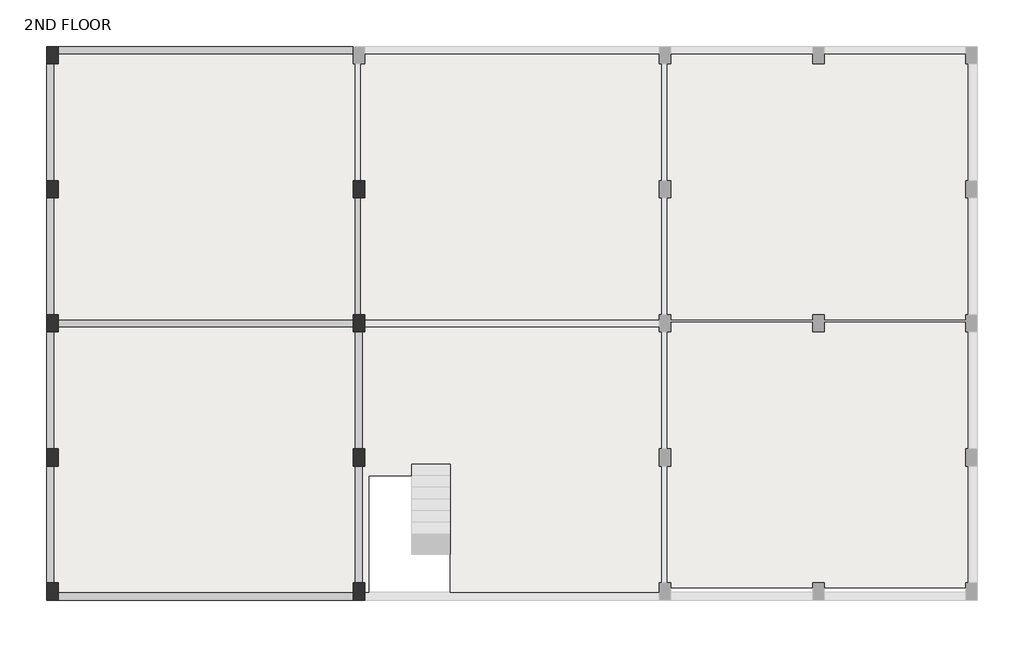
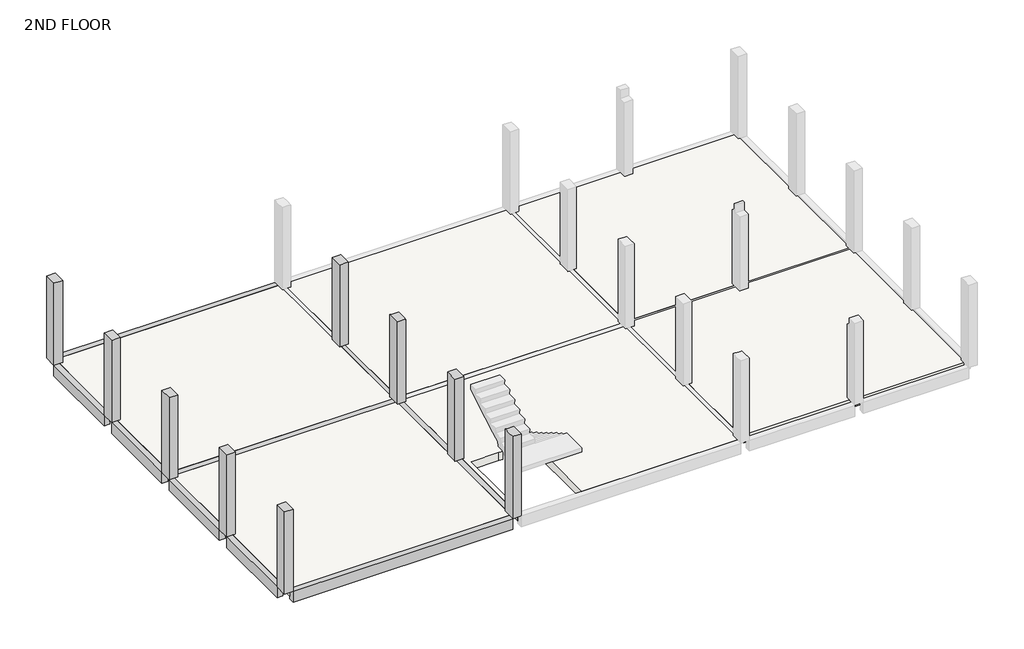
# One storey, part 1 of 2: 10 beams, 9 columns, 1 slab.
"""IFC4 building model written with IfcOpenShell, lengths in millimetres."""

from ifc_helpers import new_model, si_unit, origin, place, context, project, spatial, faceted_brep, element, save

model = new_model("IFC4")

# Units and contexts
model_context = context("Model", 3, world=origin())
ifc_project = project(units=[si_unit("LENGTHUNIT", "METRE", prefix="MILLI")], contexts=[model_context])

# Site, building, storey
site = spatial("IfcSite", under=ifc_project)
building = spatial("IfcBuilding", under=site)
storey = spatial("IfcBuildingStorey", under=building, Name="2ND FLOOR", Elevation=6096.0)

# Beams
placement = place(None, origin())
element("IfcBeam", 1, ObjectType="M_Concrete-Rectangular Beam : 200MMX400MM", at=placement, inside=storey, context=model_context, shape_type="Brep", body=[
    faceted_brep([(-3980.6874017, 15797.7008557, 6096.0), (-3980.6874017, 15997.7008557, 6096.0), (-11680.6874017, 15997.7008557, 6096.0), (-11680.6874017, 15797.7008557, 6096.0), (-3980.6874017, 15797.7008557, 5696.0), (-3980.6874017, 15797.7008557, 5796.0), (-11680.6874017, 15797.7008557, 5796.0), (-11680.6874017, 15797.7008557, 5696.0), (-3980.6874017, 15997.7008557, 5696.0), (-11680.6874017, 15997.7008557, 5696.0)], [[[0, 1, 2, 3]], [[4, 5, 0, 3, 6, 7]], [[8, 4, 7, 9]], [[1, 8, 9, 2]], [[2, 9, 7, 6, 3]], [[1, 0, 5, 4, 8]]]),
])
element("IfcBeam", 2, ObjectType="M_Concrete-Rectangular Beam : 200MMX400MM", at=placement, inside=storey, context=model_context, shape_type="Brep", body=[
    faceted_brep([(-11680.6874017, 1747.7008557, 6096.0), (-11680.6874017, 1547.7008557, 6096.0), (-3980.6874017, 1547.7008557, 6096.0), (-3980.6874017, 1747.7008557, 6096.0), (-11680.6874017, 1747.7008557, 5696.0), (-11680.6874017, 1747.7008557, 5796.0), (-3980.6874017, 1747.7008557, 5796.0), (-3980.6874017, 1747.7008557, 5696.0), (-11680.6874017, 1547.7008557, 5696.0), (-3980.6874017, 1547.7008557, 5696.0)], [[[0, 1, 2, 3]], [[4, 5, 0, 3, 6, 7]], [[8, 4, 7, 9]], [[1, 8, 9, 2]], [[1, 0, 5, 4, 8]], [[2, 9, 7, 6, 3]]]),
])
element("IfcBeam", 3, ObjectType="M_Concrete-Rectangular Beam : 200MMX400MM", at=placement, inside=storey, context=model_context, shape_type="Brep", body=[
    faceted_brep([(-3980.6874017, 8872.7008557, 6096.0), (-11680.6874017, 8872.7008557, 6096.0), (-11680.6874017, 8672.7008557, 6096.0), (-3980.6874017, 8672.7008557, 6096.0), (-11680.6874017, 8672.7008557, 5796.0), (-11680.6874017, 8672.7008557, 5696.0), (-3980.6874017, 8672.7008557, 5696.0), (-3980.6874017, 8672.7008557, 5796.0), (-11680.6874017, 8872.7008557, 5696.0), (-3980.6874017, 8872.7008557, 5696.0), (-3980.6874017, 8872.7008557, 5796.0), (-11680.6874017, 8872.7008557, 5796.0)], [[[0, 1, 2, 3]], [[3, 2, 4, 5, 6, 7]], [[6, 5, 8, 9]], [[1, 0, 10, 9, 8, 11]], [[8, 5, 4, 2, 1, 11]], [[0, 3, 7, 6, 9, 10]]]),
])
element("IfcBeam", 4, ObjectType="M_Concrete-Rectangular Beam : 200MMX400MM", at=placement, inside=storey, context=model_context, shape_type="Brep", body=[
    faceted_brep([(-11980.6874017, 12497.7008557, 6096.0), (-11780.6874017, 12497.7008557, 6096.0), (-11780.6874017, 15547.7008557, 6096.0), (-11980.6874017, 15547.7008557, 6096.0), (-11980.6874017, 12497.7008557, 5696.0), (-11980.6874017, 15547.7008557, 5696.0), (-11780.6874017, 12497.7008557, 5696.0), (-11780.6874017, 15547.7008557, 5696.0), (-11780.6874017, 12497.7008557, 5796.0), (-11780.6874017, 15547.7008557, 5796.0)], [[[0, 1, 2, 3]], [[4, 0, 3, 5]], [[6, 4, 5, 7]], [[1, 8, 6, 7, 9, 2]], [[2, 9, 7, 5, 3]], [[1, 0, 4, 6, 8]]]),
])
element("IfcBeam", 5, ObjectType="M_Concrete-Rectangular Beam : 200MMX400MM", at=placement, inside=storey, context=model_context, shape_type="Brep", body=[
    faceted_brep([(-11980.6874017, 8997.7008557, 6096.0), (-11780.6874017, 8997.7008557, 6096.0), (-11780.6874017, 12047.7008557, 6096.0), (-11980.6874017, 12047.7008557, 6096.0), (-11980.6874017, 8997.7008557, 5696.0), (-11980.6874017, 12047.7008557, 5696.0), (-11780.6874017, 8997.7008557, 5696.0), (-11780.6874017, 12047.7008557, 5696.0), (-11780.6874017, 8997.7008557, 5796.0), (-11780.6874017, 12047.7008557, 5796.0)], [[[0, 1, 2, 3]], [[4, 0, 3, 5]], [[6, 4, 5, 7]], [[1, 8, 6, 7, 9, 2]], [[1, 0, 4, 6, 8]], [[2, 9, 7, 5, 3]]]),
])
element("IfcBeam", 6, ObjectType="M_Concrete-Rectangular Beam : 200MMX400MM", at=placement, inside=storey, context=model_context, shape_type="Brep", body=[
    faceted_brep([(-11980.6874017, 5497.7008557, 6096.0), (-11780.6874017, 5497.7008557, 6096.0), (-11780.6874017, 8547.7008557, 6096.0), (-11980.6874017, 8547.7008557, 6096.0), (-11980.6874017, 5497.7008557, 5696.0), (-11980.6874017, 8547.7008557, 5696.0), (-11780.6874017, 5497.7008557, 5696.0), (-11780.6874017, 8547.7008557, 5696.0), (-11780.6874017, 5497.7008557, 5796.0), (-11780.6874017, 8547.7008557, 5796.0)], [[[0, 1, 2, 3]], [[4, 0, 3, 5]], [[6, 4, 5, 7]], [[1, 8, 6, 7, 9, 2]], [[2, 9, 7, 5, 3]], [[1, 0, 4, 6, 8]]]),
])
element("IfcBeam", 7, ObjectType="M_Concrete-Rectangular Beam : 200MMX400MM", at=placement, inside=storey, context=model_context, shape_type="Brep", body=[
    faceted_brep([(-11980.6874017, 1997.7008557, 6096.0), (-11780.6874017, 1997.7008557, 6096.0), (-11780.6874017, 5047.7008557, 6096.0), (-11980.6874017, 5047.7008557, 6096.0), (-11980.6874017, 1997.7008557, 5696.0), (-11980.6874017, 5047.7008557, 5696.0), (-11780.6874017, 1997.7008557, 5696.0), (-11780.6874017, 5047.7008557, 5696.0), (-11780.6874017, 1997.7008557, 5796.0), (-11780.6874017, 5047.7008557, 5796.0)], [[[0, 1, 2, 3]], [[4, 0, 3, 5]], [[6, 4, 5, 7]], [[1, 8, 6, 7, 9, 2]], [[1, 0, 4, 6, 8]], [[2, 9, 7, 5, 3]]]),
])
element("IfcBeam", 8, ObjectType="M_Concrete-Rectangular Beam : 200MMX400MM", at=placement, inside=storey, context=model_context, shape_type="Brep", body=[
    faceted_brep([(-3930.6874017, 5047.7008557, 6096.0), (-3930.6874017, 1997.7008557, 6096.0), (-3730.6874017, 1997.7008557, 6096.0), (-3730.6874017, 5047.7008557, 6096.0), (-3730.6874017, 1997.7008557, 5796.0), (-3730.6874017, 1997.7008557, 5696.0), (-3730.6874017, 5047.7008557, 5696.0), (-3730.6874017, 5047.7008557, 5796.0), (-3930.6874017, 1997.7008557, 5696.0), (-3930.6874017, 5047.7008557, 5696.0), (-3930.6874017, 5047.7008557, 5796.0), (-3930.6874017, 1997.7008557, 5796.0)], [[[0, 1, 2, 3]], [[3, 2, 4, 5, 6, 7]], [[6, 5, 8, 9]], [[1, 0, 10, 9, 8, 11]], [[8, 5, 4, 2, 1, 11]], [[0, 3, 7, 6, 9, 10]]]),
])
element("IfcBeam", 9, ObjectType="M_Concrete-Rectangular Beam : 200MMX400MM", at=placement, inside=storey, context=model_context, shape_type="Brep", body=[
    faceted_brep([(-3930.6874017, 8547.7008557, 6096.0), (-3930.6874017, 5497.7008557, 6096.0), (-3730.6874017, 5497.7008557, 6096.0), (-3730.6874017, 8547.7008557, 6096.0), (-3730.6874017, 5497.7008557, 5796.0), (-3730.6874017, 5497.7008557, 5696.0), (-3730.6874017, 8547.7008557, 5696.0), (-3730.6874017, 8547.7008557, 5796.0), (-3930.6874017, 5497.7008557, 5696.0), (-3930.6874017, 8547.7008557, 5696.0), (-3930.6874017, 8547.7008557, 5796.0), (-3930.6874017, 5497.7008557, 5796.0)], [[[0, 1, 2, 3]], [[3, 2, 4, 5, 6, 7]], [[6, 5, 8, 9]], [[1, 0, 10, 9, 8, 11]], [[0, 3, 7, 6, 9, 10]], [[8, 5, 4, 2, 1, 11]]]),
])
element("IfcBeam", 10, ObjectType="M_Concrete-Rectangular Beam : 200MMX400MM", at=placement, inside=storey, context=model_context, shape_type="Brep", body=[
    faceted_brep([(-3930.6874017, 12047.7008557, 6096.0), (-3930.6874017, 8997.7008557, 6096.0), (-3780.6874017, 8997.7008557, 6096.0), (-3780.6874017, 12047.7008557, 6096.0), (-3730.6874017, 8997.7008557, 5696.0), (-3730.6874017, 12047.7008557, 5696.0), (-3730.6874017, 12047.7008557, 5796.0), (-3730.6874017, 8997.7008557, 5796.0), (-3930.6874017, 8997.7008557, 5696.0), (-3930.6874017, 12047.7008557, 5696.0), (-3930.6874017, 12047.7008557, 5796.0), (-3930.6874017, 8997.7008557, 5796.0), (-3780.6874017, 12047.7008557, 5796.0), (-3780.6874017, 8997.7008557, 5796.0)], [[[0, 1, 2, 3]], [[4, 5, 6, 7]], [[5, 4, 8, 9]], [[1, 0, 10, 9, 8, 11]], [[5, 9, 10, 0, 3, 12, 6]], [[8, 4, 7, 13, 2, 1, 11]], [[12, 13, 7, 6]], [[13, 12, 3, 2]]]),
])

# Columns
element("IfcColumn", 11, ObjectType="M_Concrete-Rectangular-Column : 300 x 450mm", at=placement, inside=storey, context=model_context, shape_type="Brep", body=[
    faceted_brep([(-11680.6874017, 15997.7008557, 6096.0), (-11680.6874017, 15547.7008557, 6096.0), (-11980.6874017, 15547.7008557, 6096.0), (-11980.6874017, 15997.7008557, 6096.0), (-11680.6874017, 15997.7008557, 9144.0), (-11680.6874017, 15797.7008557, 9144.0), (-11680.6874017, 15547.7008557, 9144.0), (-11680.6874017, 15547.7008557, 8844.0), (-11780.6874017, 15547.7008557, 9144.0), (-11980.6874017, 15547.7008557, 9144.0), (-11980.6874017, 15997.7008557, 9144.0)], [[[0, 1, 2, 3]], [[1, 0, 4, 5, 6, 7]], [[2, 1, 7, 6, 8, 9]], [[3, 2, 9, 10]], [[0, 3, 10, 4]], [[10, 9, 8, 6, 5, 4]]]),
])
element("IfcColumn", 12, ObjectType="M_Concrete-Rectangular-Column : 300 x 450mm", at=placement, inside=storey, context=model_context, shape_type="Brep", body=[
    faceted_brep([(-11680.6874017, 8997.7008557, 6096.0), (-11680.6874017, 8547.7008557, 6096.0), (-11980.6874017, 8547.7008557, 6096.0), (-11980.6874017, 8997.7008557, 6096.0), (-11680.6874017, 8997.7008557, 8844.0), (-11680.6874017, 8997.7008557, 9144.0), (-11680.6874017, 8872.7008557, 9144.0), (-11680.6874017, 8672.7008557, 9144.0), (-11680.6874017, 8547.7008557, 9144.0), (-11680.6874017, 8547.7008557, 8844.0), (-11780.6874017, 8547.7008557, 9144.0), (-11980.6874017, 8547.7008557, 9144.0), (-11980.6874017, 8997.7008557, 9144.0), (-11780.6874017, 8997.7008557, 9144.0)], [[[0, 1, 2, 3]], [[1, 0, 4, 5, 6, 7, 8, 9]], [[2, 1, 9, 8, 10, 11]], [[3, 2, 11, 12]], [[0, 3, 12, 13, 5, 4]], [[12, 11, 10, 8, 7, 6, 5, 13]]]),
])
element("IfcColumn", 13, ObjectType="M_Concrete-Rectangular-Column : 300 x 450mm", at=placement, inside=storey, context=model_context, shape_type="Brep", body=[
    faceted_brep([(-11680.6874017, 1997.7008557, 6096.0), (-11680.6874017, 1547.7008557, 6096.0), (-11980.6874017, 1547.7008557, 6096.0), (-11980.6874017, 1997.7008557, 6096.0), (-11680.6874017, 1997.7008557, 8844.0), (-11680.6874017, 1997.7008557, 9144.0), (-11680.6874017, 1747.7008557, 9144.0), (-11680.6874017, 1547.7008557, 9144.0), (-11980.6874017, 1547.7008557, 9144.0), (-11980.6874017, 1997.7008557, 9144.0), (-11780.6874017, 1997.7008557, 9144.0)], [[[0, 1, 2, 3]], [[1, 0, 4, 5, 6, 7]], [[2, 1, 7, 8]], [[3, 2, 8, 9]], [[0, 3, 9, 10, 5, 4]], [[8, 7, 6, 5, 10, 9]]]),
])
element("IfcColumn", 14, ObjectType="M_Concrete-Rectangular-Column : 300 x 450mm", at=placement, inside=storey, context=model_context, shape_type="Brep", body=[
    faceted_brep([(-3680.6874017, 12497.7008557, 6096.0), (-3680.6874017, 12047.7008557, 6096.0), (-3980.6874017, 12047.7008557, 6096.0), (-3980.6874017, 12497.7008557, 6096.0), (-3680.6874017, 12497.7008557, 8844.0), (-3680.6874017, 12497.7008557, 9144.0), (-3680.6874017, 12047.7008557, 9144.0), (-3680.6874017, 12047.7008557, 8844.0), (-3780.6874017, 12047.7008557, 9144.0), (-3930.6874017, 12047.7008557, 9144.0), (-3980.6874017, 12047.7008557, 9144.0), (-3980.6874017, 12047.7008557, 8844.0), (-3980.6874017, 12497.7008557, 9144.0), (-3980.6874017, 12497.7008557, 8844.0), (-3930.6874017, 12497.7008557, 9144.0), (-3780.6874017, 12497.7008557, 9144.0)], [[[0, 1, 2, 3]], [[1, 0, 4, 5, 6, 7]], [[2, 1, 7, 6, 8, 9, 10, 11]], [[3, 2, 11, 10, 12, 13]], [[0, 3, 13, 12, 14, 15, 5, 4]], [[6, 5, 15, 14, 12, 10, 9, 8]]]),
])
element("IfcColumn", 15, ObjectType="M_Concrete-Rectangular-Column : 300 x 450mm", at=placement, inside=storey, context=model_context, shape_type="Brep", body=[
    faceted_brep([(-3680.6874017, 8997.7008557, 6096.0), (-3680.6874017, 8547.7008557, 6096.0), (-3980.6874017, 8547.7008557, 6096.0), (-3980.6874017, 8997.7008557, 6096.0), (-3680.6874017, 8997.7008557, 8844.0), (-3680.6874017, 8997.7008557, 9144.0), (-3680.6874017, 8872.7008557, 9144.0), (-3680.6874017, 8672.7008557, 9144.0), (-3680.6874017, 8547.7008557, 9144.0), (-3680.6874017, 8547.7008557, 8844.0), (-3730.6874017, 8547.7008557, 9144.0), (-3930.6874017, 8547.7008557, 9144.0), (-3980.6874017, 8547.7008557, 9144.0), (-3980.6874017, 8547.7008557, 8844.0), (-3980.6874017, 8672.7008557, 9144.0), (-3980.6874017, 8872.7008557, 9144.0), (-3980.6874017, 8997.7008557, 9144.0), (-3980.6874017, 8997.7008557, 8844.0), (-3930.6874017, 8997.7008557, 9144.0), (-3780.6874017, 8997.7008557, 9144.0)], [[[0, 1, 2, 3]], [[1, 0, 4, 5, 6, 7, 8, 9]], [[2, 1, 9, 8, 10, 11, 12, 13]], [[3, 2, 13, 12, 14, 15, 16, 17]], [[0, 3, 17, 16, 18, 19, 5, 4]], [[18, 16, 15, 14, 12, 11, 10, 8, 7, 6, 5, 19]]]),
])
element("IfcColumn", 16, ObjectType="M_Concrete-Rectangular-Column : 300 x 450mm", at=placement, inside=storey, context=model_context, shape_type="Brep", body=[
    faceted_brep([(-3680.6874017, 5497.7008557, 6096.0), (-3680.6874017, 5047.7008557, 6096.0), (-3980.6874017, 5047.7008557, 6096.0), (-3980.6874017, 5497.7008557, 6096.0), (-3680.6874017, 5497.7008557, 8844.0), (-3680.6874017, 5497.7008557, 9144.0), (-3680.6874017, 5047.7008557, 9144.0), (-3680.6874017, 5047.7008557, 8844.0), (-3730.6874017, 5047.7008557, 9144.0), (-3930.6874017, 5047.7008557, 9144.0), (-3980.6874017, 5047.7008557, 9144.0), (-3980.6874017, 5047.7008557, 8844.0), (-3980.6874017, 5497.7008557, 9144.0), (-3980.6874017, 5497.7008557, 8844.0), (-3930.6874017, 5497.7008557, 9144.0), (-3730.6874017, 5497.7008557, 9144.0)], [[[0, 1, 2, 3]], [[1, 0, 4, 5, 6, 7]], [[2, 1, 7, 6, 8, 9, 10, 11]], [[3, 2, 11, 10, 12, 13]], [[0, 3, 13, 12, 14, 15, 5, 4]], [[6, 5, 15, 14, 12, 10, 9, 8]]]),
])
element("IfcColumn", 17, ObjectType="M_Concrete-Rectangular-Column : 300 x 450mm", at=placement, inside=storey, context=model_context, shape_type="Brep", body=[
    faceted_brep([(-3680.6874017, 1997.7008557, 6096.0), (-3680.6874017, 1547.7008557, 6096.0), (-3980.6874017, 1547.7008557, 6096.0), (-3980.6874017, 1997.7008557, 6096.0), (-3680.6874017, 1997.7008557, 8844.0), (-3680.6874017, 1997.7008557, 9144.0), (-3680.6874017, 1747.7008557, 9144.0), (-3680.6874017, 1547.7008557, 9144.0), (-3980.6874017, 1547.7008557, 9144.0), (-3980.6874017, 1747.7008557, 9144.0), (-3980.6874017, 1997.7008557, 9144.0), (-3980.6874017, 1997.7008557, 8844.0), (-3930.6874017, 1997.7008557, 9144.0), (-3730.6874017, 1997.7008557, 9144.0)], [[[0, 1, 2, 3]], [[1, 0, 4, 5, 6, 7]], [[2, 1, 7, 8]], [[3, 2, 8, 9, 10, 11]], [[0, 3, 11, 10, 12, 13, 5, 4]], [[8, 7, 6, 5, 13, 12, 10, 9]]]),
])
element("IfcColumn", 18, ObjectType="M_Concrete-Rectangular-Column : 300 x 450mm", at=placement, inside=storey, context=model_context, shape_type="Brep", body=[
    faceted_brep([(-11680.6874017, 12497.7008557, 6096.0), (-11680.6874017, 12047.7008557, 6096.0), (-11980.6874017, 12047.7008557, 6096.0), (-11980.6874017, 12497.7008557, 6096.0), (-11680.6874017, 12497.7008557, 8844.0), (-11680.6874017, 12497.7008557, 9144.0), (-11680.6874017, 12047.7008557, 9144.0), (-11680.6874017, 12047.7008557, 8844.0), (-11780.6874017, 12047.7008557, 9144.0), (-11980.6874017, 12047.7008557, 9144.0), (-11980.6874017, 12497.7008557, 9144.0), (-11780.6874017, 12497.7008557, 9144.0)], [[[0, 1, 2, 3]], [[1, 0, 4, 5, 6, 7]], [[2, 1, 7, 6, 8, 9]], [[3, 2, 9, 10]], [[0, 3, 10, 11, 5, 4]], [[6, 5, 11, 10, 9, 8]]]),
])
element("IfcColumn", 19, ObjectType="M_Concrete-Rectangular-Column : 300 x 450mm", at=placement, inside=storey, context=model_context, shape_type="Brep", body=[
    faceted_brep([(-11680.6874017, 5497.7008557, 6096.0), (-11680.6874017, 5047.7008557, 6096.0), (-11980.6874017, 5047.7008557, 6096.0), (-11980.6874017, 5497.7008557, 6096.0), (-11680.6874017, 5497.7008557, 8844.0), (-11680.6874017, 5497.7008557, 9144.0), (-11680.6874017, 5047.7008557, 9144.0), (-11680.6874017, 5047.7008557, 8844.0), (-11780.6874017, 5047.7008557, 9144.0), (-11980.6874017, 5047.7008557, 9144.0), (-11980.6874017, 5497.7008557, 9144.0), (-11780.6874017, 5497.7008557, 9144.0)], [[[0, 1, 2, 3]], [[1, 0, 4, 5, 6, 7]], [[2, 1, 7, 6, 8, 9]], [[3, 2, 9, 10]], [[0, 3, 10, 11, 5, 4]], [[6, 5, 11, 10, 9, 8]]]),
])

# Slab
element("IfcSlab", 20, ObjectType="Generic 300mm", at=placement, inside=storey, context=model_context, shape_type="Brep", body=[
    faceted_brep([(-11680.6874017, 15547.7008557, 5796.0), (-11680.6874017, 15797.7008557, 5796.0), (-3980.6874017, 15797.7008557, 5796.0), (-3980.6874017, 15547.7008557, 5796.0), (-3930.6874017, 15547.7008557, 5796.0), (-3930.6874017, 12497.7008557, 5796.0), (-3980.6874017, 12497.7008557, 5796.0), (-3980.6874017, 12047.7008557, 5796.0), (-3930.6874017, 12047.7008557, 5796.0), (-3930.6874017, 8997.7008557, 5796.0), (-3980.6874017, 8997.7008557, 5796.0), (-3980.6874017, 8872.7008557, 5796.0), (-11680.6874017, 8872.7008557, 5796.0), (-11680.6874017, 8997.7008557, 5796.0), (-11780.6874017, 8997.7008557, 5796.0), (-11780.6874017, 12047.7008557, 5796.0), (-11680.6874017, 12047.7008557, 5796.0), (-11680.6874017, 12497.7008557, 5796.0), (-11780.6874017, 12497.7008557, 5796.0), (-11780.6874017, 15547.7008557, 5796.0), (-11680.6874017, 15797.7008557, 6096.0), (-11680.6874017, 15547.7008557, 6096.0), (-11780.6874017, 15547.7008557, 6096.0), (-11780.6874017, 12497.7008557, 6096.0), (-11680.6874017, 12497.7008557, 6096.0), (-11680.6874017, 12047.7008557, 6096.0), (-11780.6874017, 12047.7008557, 6096.0), (-11780.6874017, 8997.7008557, 6096.0), (-11680.6874017, 8997.7008557, 6096.0), (-11680.6874017, 8872.7008557, 6096.0), (-3980.6874017, 8872.7008557, 6096.0), (-3980.6874017, 8997.7008557, 6096.0), (-3930.6874017, 8997.7008557, 6096.0), (-3930.6874017, 12047.7008557, 6096.0), (-3980.6874017, 12047.7008557, 6096.0), (-3980.6874017, 12497.7008557, 6096.0), (-3930.6874017, 12497.7008557, 6096.0), (-3930.6874017, 15547.7008557, 6096.0), (-3980.6874017, 15547.7008557, 6096.0), (-3980.6874017, 15797.7008557, 6096.0)], [[[0, 1, 2, 3, 4, 5, 6, 7, 8, 9, 10, 11, 12, 13, 14, 15, 16, 17, 18, 19]], [[20, 21, 22, 23, 24, 25, 26, 27, 28, 29, 30, 31, 32, 33, 34, 35, 36, 37, 38, 39]], [[1, 0, 21, 20]], [[2, 1, 20, 39]], [[3, 2, 39, 38]], [[4, 3, 38, 37]], [[5, 4, 37, 36]], [[6, 5, 36, 35]], [[7, 6, 35, 34]], [[8, 7, 34, 33]], [[9, 8, 33, 32]], [[10, 9, 32, 31]], [[11, 10, 31, 30]], [[12, 11, 30, 29]], [[13, 12, 29, 28]], [[14, 13, 28, 27]], [[15, 14, 27, 26]], [[16, 15, 26, 25]], [[17, 16, 25, 24]], [[18, 17, 24, 23]], [[19, 18, 23, 22]], [[0, 19, 22, 21]]]),
    faceted_brep([(-3680.6874017, 15547.7008557, 5796.0), (-3680.6874017, 15797.7008557, 5796.0), (4019.3125983, 15797.7008557, 5796.0), (4019.3125983, 15547.7008557, 5796.0), (4069.3125983, 15547.7008557, 5796.0), (4069.3125983, 12497.7008557, 5796.0), (4019.3125983, 12497.7008557, 5796.0), (4019.3125983, 12047.7008557, 5796.0), (4069.3125983, 12047.7008557, 5796.0), (4069.3125983, 8997.7008557, 5796.0), (4019.3125983, 8997.7008557, 5796.0), (4019.3125983, 8872.7008557, 5796.0), (-3680.6874017, 8872.7008557, 5796.0), (-3680.6874017, 8997.7008557, 5796.0), (-3730.6874017, 8997.7008557, 5796.0), (-3780.6874017, 8997.7008557, 5796.0), (-3780.6874017, 12047.7008557, 5796.0), (-3730.6874017, 12047.7008557, 5796.0), (-3680.6874017, 12047.7008557, 5796.0), (-3680.6874017, 12497.7008557, 5796.0), (-3730.6874017, 12497.7008557, 5796.0), (-3780.6874017, 12497.7008557, 5796.0), (-3780.6874017, 15547.7008557, 5796.0), (-3730.6874017, 15547.7008557, 5796.0), (-3680.6874017, 15797.7008557, 6096.0), (-3680.6874017, 15547.7008557, 6096.0), (-3780.6874017, 15547.7008557, 6096.0), (-3780.6874017, 12497.7008557, 6096.0), (-3680.6874017, 12497.7008557, 6096.0), (-3680.6874017, 12047.7008557, 6096.0), (-3780.6874017, 12047.7008557, 6096.0), (-3780.6874017, 8997.7008557, 6096.0), (-3680.6874017, 8997.7008557, 6096.0), (-3680.6874017, 8872.7008557, 6096.0), (4019.3125983, 8872.7008557, 6096.0), (4019.3125983, 8997.7008557, 6096.0), (4069.3125983, 8997.7008557, 6096.0), (4069.3125983, 12047.7008557, 6096.0), (4019.3125983, 12047.7008557, 6096.0), (4019.3125983, 12497.7008557, 6096.0), (4069.3125983, 12497.7008557, 6096.0), (4069.3125983, 15547.7008557, 6096.0), (4019.3125983, 15547.7008557, 6096.0), (4019.3125983, 15797.7008557, 6096.0)], [[[0, 1, 2, 3, 4, 5, 6, 7, 8, 9, 10, 11, 12, 13, 14, 15, 16, 17, 18, 19, 20, 21, 22, 23]], [[24, 25, 26, 27, 28, 29, 30, 31, 32, 33, 34, 35, 36, 37, 38, 39, 40, 41, 42, 43]], [[1, 0, 25, 24]], [[2, 1, 24, 43]], [[3, 2, 43, 42]], [[4, 3, 42, 41]], [[5, 4, 41, 40]], [[6, 5, 40, 39]], [[7, 6, 39, 38]], [[8, 7, 38, 37]], [[9, 8, 37, 36]], [[10, 9, 36, 35]], [[11, 10, 35, 34]], [[12, 11, 34, 33]], [[13, 12, 33, 32]], [[15, 14, 13, 32, 31]], [[16, 15, 31, 30]], [[18, 17, 16, 30, 29]], [[19, 18, 29, 28]], [[21, 20, 19, 28, 27]], [[22, 21, 27, 26]], [[0, 23, 22, 26, 25]]]),
    faceted_brep([(4319.3125983, 15547.7008557, 5796.0), (4319.3125983, 15797.7008557, 5796.0), (8019.3125983, 15797.7008557, 5796.0), (8319.3125983, 15797.7008557, 5796.0), (12019.3125983, 15797.7008557, 5796.0), (12019.3125983, 15547.7008557, 5796.0), (12069.3125983, 15547.7008557, 5796.0), (12069.3125983, 12497.7008557, 5796.0), (12019.3125983, 12497.7008557, 5796.0), (12019.3125983, 12047.7008557, 5796.0), (12069.3125983, 12047.7008557, 5796.0), (12069.3125983, 8997.7008557, 5796.0), (12019.3125983, 8997.7008557, 5796.0), (12019.3125983, 8872.7008557, 5796.0), (8319.3125983, 8872.7008557, 5796.0), (8019.3125983, 8872.7008557, 5796.0), (4319.3125983, 8872.7008557, 5796.0), (4319.3125983, 8997.7008557, 5796.0), (4269.3125983, 8997.7008557, 5796.0), (4219.3125983, 8997.7008557, 5796.0), (4219.3125983, 12047.7008557, 5796.0), (4269.3125983, 12047.7008557, 5796.0), (4319.3125983, 12047.7008557, 5796.0), (4319.3125983, 12497.7008557, 5796.0), (4269.3125983, 12497.7008557, 5796.0), (4219.3125983, 12497.7008557, 5796.0), (4219.3125983, 15547.7008557, 5796.0), (4269.3125983, 15547.7008557, 5796.0), (4319.3125983, 15797.7008557, 6096.0), (4319.3125983, 15547.7008557, 6096.0), (4219.3125983, 15547.7008557, 6096.0), (4219.3125983, 12497.7008557, 6096.0), (4319.3125983, 12497.7008557, 6096.0), (4319.3125983, 12047.7008557, 6096.0), (4219.3125983, 12047.7008557, 6096.0), (4219.3125983, 8997.7008557, 6096.0), (4319.3125983, 8997.7008557, 6096.0), (4319.3125983, 8872.7008557, 6096.0), (8019.3125983, 8872.7008557, 6096.0), (8319.3125983, 8872.7008557, 6096.0), (12019.3125983, 8872.7008557, 6096.0), (12019.3125983, 8997.7008557, 6096.0), (12069.3125983, 8997.7008557, 6096.0), (12069.3125983, 12047.7008557, 6096.0), (12019.3125983, 12047.7008557, 6096.0), (12019.3125983, 12497.7008557, 6096.0), (12069.3125983, 12497.7008557, 6096.0), (12069.3125983, 15547.7008557, 6096.0), (12019.3125983, 15547.7008557, 6096.0), (12019.3125983, 15797.7008557, 6096.0), (8319.3125983, 15797.7008557, 6096.0), (8019.3125983, 15797.7008557, 6096.0)], [[[0, 1, 2, 3, 4, 5, 6, 7, 8, 9, 10, 11, 12, 13, 14, 15, 16, 17, 18, 19, 20, 21, 22, 23, 24, 25, 26, 27]], [[28, 29, 30, 31, 32, 33, 34, 35, 36, 37, 38, 39, 40, 41, 42, 43, 44, 45, 46, 47, 48, 49, 50, 51]], [[1, 0, 29, 28]], [[4, 3, 2, 1, 28, 51, 50, 49]], [[5, 4, 49, 48]], [[6, 5, 48, 47]], [[7, 6, 47, 46]], [[8, 7, 46, 45]], [[9, 8, 45, 44]], [[10, 9, 44, 43]], [[11, 10, 43, 42]], [[12, 11, 42, 41]], [[13, 12, 41, 40]], [[16, 15, 14, 13, 40, 39, 38, 37]], [[17, 16, 37, 36]], [[19, 18, 17, 36, 35]], [[20, 19, 35, 34]], [[22, 21, 20, 34, 33]], [[23, 22, 33, 32]], [[25, 24, 23, 32, 31]], [[26, 25, 31, 30]], [[0, 27, 26, 30, 29]]]),
    faceted_brep([(-3680.6874017, 8547.7008557, 5796.0), (-3680.6874017, 8672.7008557, 5796.0), (4019.3125983, 8672.7008557, 5796.0), (4019.3125983, 8547.7008557, 5796.0), (4069.3125983, 8547.7008557, 5796.0), (4069.3125983, 5497.7008557, 5796.0), (4019.3125983, 5497.7008557, 5796.0), (4019.3125983, 5047.7008557, 5796.0), (4069.3125983, 5047.7008557, 5796.0), (4069.3125983, 1997.7008557, 5796.0), (4019.3125983, 1997.7008557, 5796.0), (4019.3125983, 1747.7008557, 5796.0), (-1437.0874017, 1747.7008557, 5796.0), (-1437.0874017, 5100.5008557, 5796.0), (-2453.0874017, 5100.5008557, 5796.0), (-2453.0874017, 4795.7008557, 5796.0), (-2593.0874017, 4795.7008557, 5796.0), (-3570.6874017, 4795.7008557, 5796.0), (-3570.6874017, 1747.7008557, 5796.0), (-3680.6874017, 1747.7008557, 5796.0), (-3680.6874017, 1997.7008557, 5796.0), (-3730.6874017, 1997.7008557, 5796.0), (-3730.6874017, 5047.7008557, 5796.0), (-3680.6874017, 5047.7008557, 5796.0), (-3680.6874017, 5497.7008557, 5796.0), (-3730.6874017, 5497.7008557, 5796.0), (-3730.6874017, 8547.7008557, 5796.0), (-3680.6874017, 8672.7008557, 6096.0), (-3680.6874017, 8547.7008557, 6096.0), (-3730.6874017, 8547.7008557, 6096.0), (-3730.6874017, 5497.7008557, 6096.0), (-3680.6874017, 5497.7008557, 6096.0), (-3680.6874017, 5047.7008557, 6096.0), (-3730.6874017, 5047.7008557, 6096.0), (-3730.6874017, 1997.7008557, 6096.0), (-3680.6874017, 1997.7008557, 6096.0), (-3680.6874017, 1747.7008557, 6096.0), (-3570.6874017, 1747.7008557, 6096.0), (-3570.6874017, 4795.7008557, 6096.0), (-2593.0874017, 4795.7008557, 6096.0), (-2453.0874017, 4795.7008557, 6096.0), (-2453.0874017, 5100.5008557, 6096.0), (-1437.0874017, 5100.5008557, 6096.0), (-1437.0874017, 1747.7008557, 6096.0), (4019.3125983, 1747.7008557, 6096.0), (4019.3125983, 1997.7008557, 6096.0), (4069.3125983, 1997.7008557, 6096.0), (4069.3125983, 5047.7008557, 6096.0), (4019.3125983, 5047.7008557, 6096.0), (4019.3125983, 5497.7008557, 6096.0), (4069.3125983, 5497.7008557, 6096.0), (4069.3125983, 8547.7008557, 6096.0), (4019.3125983, 8547.7008557, 6096.0), (4019.3125983, 8672.7008557, 6096.0)], [[[0, 1, 2, 3, 4, 5, 6, 7, 8, 9, 10, 11, 12, 13, 14, 15, 16, 17, 18, 19, 20, 21, 22, 23, 24, 25, 26]], [[27, 28, 29, 30, 31, 32, 33, 34, 35, 36, 37, 38, 39, 40, 41, 42, 43, 44, 45, 46, 47, 48, 49, 50, 51, 52, 53]], [[1, 0, 28, 27]], [[2, 1, 27, 53]], [[3, 2, 53, 52]], [[4, 3, 52, 51]], [[5, 4, 51, 50]], [[6, 5, 50, 49]], [[7, 6, 49, 48]], [[8, 7, 48, 47]], [[9, 8, 47, 46]], [[10, 9, 46, 45]], [[11, 10, 45, 44]], [[11, 44, 43, 12]], [[36, 19, 18, 37]], [[20, 19, 36, 35]], [[21, 20, 35, 34]], [[22, 21, 34, 33]], [[23, 22, 33, 32]], [[24, 23, 32, 31]], [[25, 24, 31, 30]], [[26, 25, 30, 29]], [[0, 26, 29, 28]], [[42, 13, 12, 43]], [[13, 42, 41, 14]], [[14, 41, 40, 15]], [[15, 40, 39, 16]], [[16, 39, 38, 17]], [[17, 38, 37, 18]]]),
    faceted_brep([(-3980.6874017, 1747.7008557, 5796.0), (-11680.6874017, 1747.7008557, 5796.0), (-11680.6874017, 1997.7008557, 5796.0), (-11780.6874017, 1997.7008557, 5796.0), (-11780.6874017, 5047.7008557, 5796.0), (-11680.6874017, 5047.7008557, 5796.0), (-11680.6874017, 5497.7008557, 5796.0), (-11780.6874017, 5497.7008557, 5796.0), (-11780.6874017, 8547.7008557, 5796.0), (-11680.6874017, 8547.7008557, 5796.0), (-11680.6874017, 8672.7008557, 5796.0), (-3980.6874017, 8672.7008557, 5796.0), (-3980.6874017, 8547.7008557, 5796.0), (-3930.6874017, 8547.7008557, 5796.0), (-3930.6874017, 5497.7008557, 5796.0), (-3980.6874017, 5497.7008557, 5796.0), (-3980.6874017, 5047.7008557, 5796.0), (-3930.6874017, 5047.7008557, 5796.0), (-3930.6874017, 1997.7008557, 5796.0), (-3980.6874017, 1997.7008557, 5796.0), (-11680.6874017, 1747.7008557, 6096.0), (-3980.6874017, 1747.7008557, 6096.0), (-3980.6874017, 1997.7008557, 6096.0), (-3930.6874017, 1997.7008557, 6096.0), (-3930.6874017, 5047.7008557, 6096.0), (-3980.6874017, 5047.7008557, 6096.0), (-3980.6874017, 5497.7008557, 6096.0), (-3930.6874017, 5497.7008557, 6096.0), (-3930.6874017, 8547.7008557, 6096.0), (-3980.6874017, 8547.7008557, 6096.0), (-3980.6874017, 8672.7008557, 6096.0), (-11680.6874017, 8672.7008557, 6096.0), (-11680.6874017, 8547.7008557, 6096.0), (-11780.6874017, 8547.7008557, 6096.0), (-11780.6874017, 5497.7008557, 6096.0), (-11680.6874017, 5497.7008557, 6096.0), (-11680.6874017, 5047.7008557, 6096.0), (-11780.6874017, 5047.7008557, 6096.0), (-11780.6874017, 1997.7008557, 6096.0), (-11680.6874017, 1997.7008557, 6096.0)], [[[0, 1, 2, 3, 4, 5, 6, 7, 8, 9, 10, 11, 12, 13, 14, 15, 16, 17, 18, 19]], [[20, 21, 22, 23, 24, 25, 26, 27, 28, 29, 30, 31, 32, 33, 34, 35, 36, 37, 38, 39]], [[1, 0, 21, 20]], [[2, 1, 20, 39]], [[3, 2, 39, 38]], [[4, 3, 38, 37]], [[5, 4, 37, 36]], [[6, 5, 36, 35]], [[7, 6, 35, 34]], [[8, 7, 34, 33]], [[9, 8, 33, 32]], [[10, 9, 32, 31]], [[11, 10, 31, 30]], [[12, 11, 30, 29]], [[13, 12, 29, 28]], [[14, 13, 28, 27]], [[15, 14, 27, 26]], [[16, 15, 26, 25]], [[17, 16, 25, 24]], [[18, 17, 24, 23]], [[19, 18, 23, 22]], [[0, 19, 22, 21]]]),
    faceted_brep([(4319.3125983, 8547.7008557, 5796.0), (4319.3125983, 8672.7008557, 5796.0), (4319.3125983, 8797.7008557, 5796.0), (8019.3125983, 8797.7008557, 5796.0), (8319.3125983, 8797.7008557, 5796.0), (12019.3125983, 8797.7008557, 5796.0), (12019.3125983, 8672.7008557, 5796.0), (12019.3125983, 8547.7008557, 5796.0), (12069.3125983, 8547.7008557, 5796.0), (12069.3125983, 5497.7008557, 5796.0), (12019.3125983, 5497.7008557, 5796.0), (12019.3125983, 5047.7008557, 5796.0), (12069.3125983, 5047.7008557, 5796.0), (12069.3125983, 1997.7008557, 5796.0), (12019.3125983, 1997.7008557, 5796.0), (12019.3125983, 1872.7008557, 5796.0), (8319.3125983, 1872.7008557, 5796.0), (8019.3125983, 1872.7008557, 5796.0), (4319.3125983, 1872.7008557, 5796.0), (4319.3125983, 1997.7008557, 5796.0), (4269.3125983, 1997.7008557, 5796.0), (4219.3125983, 1997.7008557, 5796.0), (4219.3125983, 5047.7008557, 5796.0), (4269.3125983, 5047.7008557, 5796.0), (4319.3125983, 5047.7008557, 5796.0), (4319.3125983, 5497.7008557, 5796.0), (4269.3125983, 5497.7008557, 5796.0), (4219.3125983, 5497.7008557, 5796.0), (4219.3125983, 8547.7008557, 5796.0), (4269.3125983, 8547.7008557, 5796.0), (4319.3125983, 8797.7008557, 6096.0), (4319.3125983, 8547.7008557, 6096.0), (4219.3125983, 8547.7008557, 6096.0), (4219.3125983, 5497.7008557, 6096.0), (4319.3125983, 5497.7008557, 6096.0), (4319.3125983, 5047.7008557, 6096.0), (4219.3125983, 5047.7008557, 6096.0), (4219.3125983, 1997.7008557, 6096.0), (4319.3125983, 1997.7008557, 6096.0), (4319.3125983, 1872.7008557, 6096.0), (8019.3125983, 1872.7008557, 6096.0), (8319.3125983, 1872.7008557, 6096.0), (12019.3125983, 1872.7008557, 6096.0), (12019.3125983, 1997.7008557, 6096.0), (12069.3125983, 1997.7008557, 6096.0), (12069.3125983, 5047.7008557, 6096.0), (12019.3125983, 5047.7008557, 6096.0), (12019.3125983, 5497.7008557, 6096.0), (12069.3125983, 5497.7008557, 6096.0), (12069.3125983, 8547.7008557, 6096.0), (12019.3125983, 8547.7008557, 6096.0), (12019.3125983, 8797.7008557, 6096.0), (8319.3125983, 8797.7008557, 6096.0), (8019.3125983, 8797.7008557, 6096.0)], [[[0, 1, 2, 3, 4, 5, 6, 7, 8, 9, 10, 11, 12, 13, 14, 15, 16, 17, 18, 19, 20, 21, 22, 23, 24, 25, 26, 27, 28, 29]], [[30, 31, 32, 33, 34, 35, 36, 37, 38, 39, 40, 41, 42, 43, 44, 45, 46, 47, 48, 49, 50, 51, 52, 53]], [[2, 1, 0, 31, 30]], [[5, 4, 3, 2, 30, 53, 52, 51]], [[7, 6, 5, 51, 50]], [[8, 7, 50, 49]], [[9, 8, 49, 48]], [[10, 9, 48, 47]], [[11, 10, 47, 46]], [[12, 11, 46, 45]], [[13, 12, 45, 44]], [[14, 13, 44, 43]], [[15, 14, 43, 42]], [[18, 17, 16, 15, 42, 41, 40, 39]], [[19, 18, 39, 38]], [[21, 20, 19, 38, 37]], [[22, 21, 37, 36]], [[24, 23, 22, 36, 35]], [[25, 24, 35, 34]], [[27, 26, 25, 34, 33]], [[28, 27, 33, 32]], [[0, 29, 28, 32, 31]]]),
])

save(model, "model.ifc")

# Revit data of these elements
# Type "M_Concrete-Rectangular Beam : 200MMX400MM"
#   Length [instance default] = 5' - 0"
#   b = 0' - 7.87402"
#   h = 1' - 3.74803"
#   Structural Material [instance default] = Concrete, Cast-in-Place gray
#   Assembly Code = ""
# Type "M_Concrete-Rectangular-Column : 300 x 450mm"
#   b = 0' - 11.81102"
#   h = 1' - 5.71654"
#   Structural Material [instance default] = Concrete, Cast-in-Place gray
# Type "Generic 300mm"
#   Function = 0
#   Layers, outside or top first: 0' - 11.81102" no material (function 1)
# Elements 1, 2, 3, 4, 5, 6, 7, 8, 9, 10 (IfcBeam, "M_Concrete-Rectangular Beam : 200MMX400MM")
#   Structural Material = Concrete, Cast-in-Place gray
#   Phase Created = New Construction
#   Materials on its faces: "Concrete, Cast-in-Place gray"
# Elements 11, 12, 13, 14, 15, 16, 17, 18, 19 (IfcColumn, "M_Concrete-Rectangular-Column : 300 x 450mm")
#   Structural Material = Concrete, Cast-in-Place gray
#   Phase Created = New Construction
#   Materials on its faces: "Concrete, Cast-in-Place gray"
# Element 20 (IfcSlab, "Generic 300mm")
#   Height Offset From Level = 0' - 0"
#   built-in parameter 1001954 = 1
#   Phase Created = New Construction
#   Materials on its faces: "Default Floor"
# Materials
#   "Concrete, Cast-in-Place gray": class "Concrete", colour RGB 192 192 192, transparency 0, Description = "Cast-in-place concrete", Cost = 0
#   "Default Floor": colour RGB 127 127 127, transparency 0, Cost = 0
